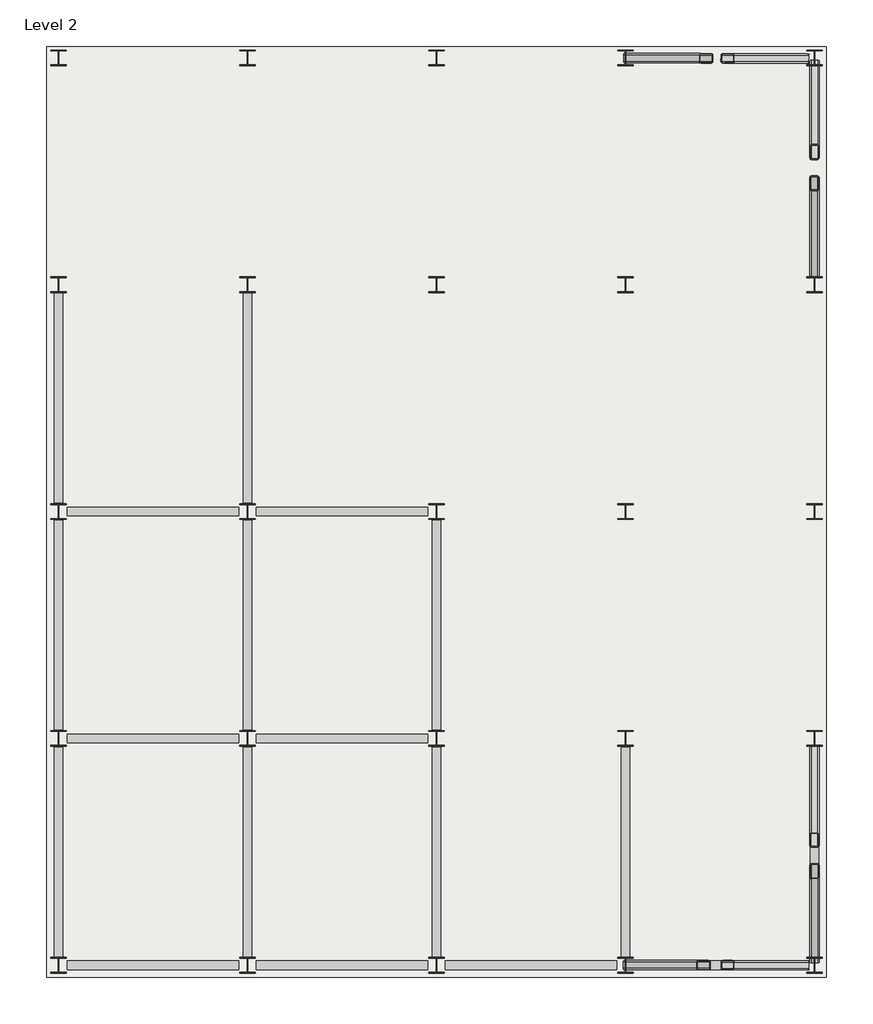
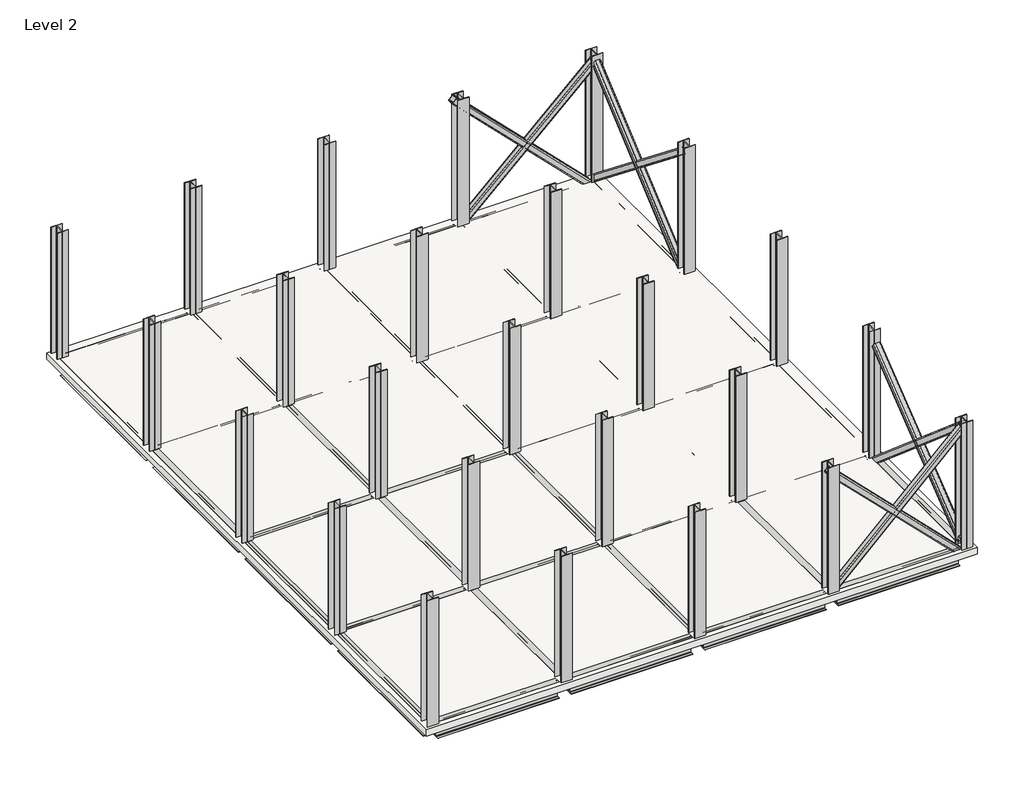
# One storey: 40 beams, 25 columns, 8 members, 1 slab.
"""IFC4 building model written with IfcOpenShell, lengths in millimetres."""

from ifc_helpers import new_model, si_unit, frame, origin, place, context, project, spatial, polyline, outline, extrude, transform, mapped, element, save
from components import w_shapes_w16x26_71b85d0e, w_shapes_w16x26_5730d789, w_shapes_column_w10x49_ceff5d29, hss_square_hss6x6x1_2_008024fe, hss_square_hss6x6x1_2_7c43692b, hss_square_hss6x6x1_2_5f011b37, hss_square_hss6x6x1_2_b9926e2d, hss_square_hss6x6x1_2_e6555cf9, hss_square_hss6x6x1_2_f7a49a43, hss_square_hss6x6x1_2_10b7330d, hss_square_hss6x6x1_2_f3b36863

model = new_model("IFC4")

# Units and contexts
model_context = context("Model", 3, world=origin())
ifc_project = project(units=[si_unit("LENGTHUNIT", "METRE", prefix="MILLI")], contexts=[model_context])

# Site, building, storey
site = spatial("IfcSite", under=ifc_project)
building = spatial("IfcBuilding", under=site)
storey = spatial("IfcBuildingStorey", under=building, Name="Level 2", Elevation=3048.0)

# Beams
placement = place(None, origin())
w_shapes_w16x26_shape = w_shapes_w16x26_71b85d0e(model_context)
element("IfcBeam", 1, ObjectType="W Shapes : W16X26", at=placement, inside=storey, context=model_context, shape_type="MappedRepresentation", body=[
    mapped(w_shapes_w16x26_shape, transform((-5883.5186598, -2213.7239423, 2848.61), x_axis=(1.0, 0.0, 0.0), y_axis=(0.0, 1.0, 0.0), z_axis=(0.0, 0.0, 1.0))),
])
element("IfcBeam", 2, ObjectType="W Shapes : W16X26", at=placement, inside=storey, context=model_context, shape_type="MappedRepresentation", body=[
    mapped(w_shapes_w16x26_shape, transform((-2835.5186598, -2213.7239423, 2848.61), x_axis=(1.0, 0.0, 0.0), y_axis=(0.0, 1.0, 0.0), z_axis=(0.0, 0.0, 1.0))),
])
element("IfcBeam", 3, ObjectType="W Shapes : W16X26", at=placement, inside=storey, context=model_context, shape_type="MappedRepresentation", body=[
    mapped(w_shapes_w16x26_shape, transform((212.4813402, -2213.7239423, 2848.61), x_axis=(1.0, 0.0, 0.0), y_axis=(0.0, 1.0, 0.0), z_axis=(0.0, 0.0, 1.0))),
])
element("IfcBeam", 4, ObjectType="W Shapes : W16X26", at=placement, inside=storey, context=model_context, shape_type="MappedRepresentation", body=[
    mapped(w_shapes_w16x26_shape, transform((3260.4813402, -2213.7239423, 2848.61), x_axis=(1.0, 0.0, 0.0), y_axis=(0.0, 1.0, 0.0), z_axis=(0.0, 0.0, 1.0))),
])
element("IfcBeam", 5, ObjectType="W Shapes : W16X26", at=placement, inside=storey, context=model_context, shape_type="MappedRepresentation", body=[
    mapped(w_shapes_w16x26_shape, transform((-5883.5186598, 1443.8760577, 2848.61), x_axis=(1.0, 0.0, 0.0), y_axis=(0.0, 1.0, 0.0), z_axis=(0.0, 0.0, 1.0))),
])
element("IfcBeam", 6, ObjectType="W Shapes : W16X26", at=placement, inside=storey, context=model_context, shape_type="MappedRepresentation", body=[
    mapped(w_shapes_w16x26_shape, transform((-2835.5186598, 1443.8760577, 2848.61), x_axis=(1.0, 0.0, 0.0), y_axis=(0.0, 1.0, 0.0), z_axis=(0.0, 0.0, 1.0))),
])
element("IfcBeam", 7, ObjectType="W Shapes : W16X26", at=placement, inside=storey, context=model_context, shape_type="MappedRepresentation", body=[
    mapped(w_shapes_w16x26_shape, transform((212.4813402, 1443.8760577, 2848.61), x_axis=(1.0, 0.0, 0.0), y_axis=(0.0, 1.0, 0.0), z_axis=(0.0, 0.0, 1.0))),
])
element("IfcBeam", 8, ObjectType="W Shapes : W16X26", at=placement, inside=storey, context=model_context, shape_type="MappedRepresentation", body=[
    mapped(w_shapes_w16x26_shape, transform((3260.4813402, 1443.8760577, 2848.61), x_axis=(1.0, 0.0, 0.0), y_axis=(0.0, 1.0, 0.0), z_axis=(0.0, 0.0, 1.0))),
])
element("IfcBeam", 9, ObjectType="W Shapes : W16X26", at=placement, inside=storey, context=model_context, shape_type="MappedRepresentation", body=[
    mapped(w_shapes_w16x26_shape, transform((-5883.5186598, 5101.4760577, 2848.61), x_axis=(1.0, 0.0, 0.0), y_axis=(0.0, 1.0, 0.0), z_axis=(0.0, 0.0, 1.0))),
])
element("IfcBeam", 10, ObjectType="W Shapes : W16X26", at=placement, inside=storey, context=model_context, shape_type="MappedRepresentation", body=[
    mapped(w_shapes_w16x26_shape, transform((-2835.5186598, 5101.4760577, 2848.61), x_axis=(1.0, 0.0, 0.0), y_axis=(0.0, 1.0, 0.0), z_axis=(0.0, 0.0, 1.0))),
])
element("IfcBeam", 11, ObjectType="W Shapes : W16X26", at=placement, inside=storey, context=model_context, shape_type="MappedRepresentation", body=[
    mapped(w_shapes_w16x26_shape, transform((212.4813402, 5101.4760577, 2848.61), x_axis=(1.0, 0.0, 0.0), y_axis=(0.0, 1.0, 0.0), z_axis=(0.0, 0.0, 1.0))),
])
element("IfcBeam", 12, ObjectType="W Shapes : W16X26", at=placement, inside=storey, context=model_context, shape_type="MappedRepresentation", body=[
    mapped(w_shapes_w16x26_shape, transform((3260.4813402, 5101.4760577, 2848.61), x_axis=(1.0, 0.0, 0.0), y_axis=(0.0, 1.0, 0.0), z_axis=(0.0, 0.0, 1.0))),
])
element("IfcBeam", 13, ObjectType="W Shapes : W16X26", at=placement, inside=storey, context=model_context, shape_type="MappedRepresentation", body=[
    mapped(w_shapes_w16x26_shape, transform((-5883.5186598, 8759.0760577, 2848.61), x_axis=(1.0, 0.0, 0.0), y_axis=(0.0, 1.0, 0.0), z_axis=(0.0, 0.0, 1.0))),
])
element("IfcBeam", 14, ObjectType="W Shapes : W16X26", at=placement, inside=storey, context=model_context, shape_type="MappedRepresentation", body=[
    mapped(w_shapes_w16x26_shape, transform((-2835.5186598, 8759.0760577, 2848.61), x_axis=(1.0, 0.0, 0.0), y_axis=(0.0, 1.0, 0.0), z_axis=(0.0, 0.0, 1.0))),
])
element("IfcBeam", 15, ObjectType="W Shapes : W16X26", at=placement, inside=storey, context=model_context, shape_type="MappedRepresentation", body=[
    mapped(w_shapes_w16x26_shape, transform((212.4813402, 8759.0760577, 2848.61), x_axis=(1.0, 0.0, 0.0), y_axis=(0.0, 1.0, 0.0), z_axis=(0.0, 0.0, 1.0))),
])
element("IfcBeam", 16, ObjectType="W Shapes : W16X26", at=placement, inside=storey, context=model_context, shape_type="MappedRepresentation", body=[
    mapped(w_shapes_w16x26_shape, transform((3260.4813402, 8759.0760577, 2848.61), x_axis=(1.0, 0.0, 0.0), y_axis=(0.0, 1.0, 0.0), z_axis=(0.0, 0.0, 1.0))),
])
element("IfcBeam", 17, ObjectType="W Shapes : W16X26", at=placement, inside=storey, context=model_context, shape_type="MappedRepresentation", body=[
    mapped(w_shapes_w16x26_shape, transform((-5883.5186598, 12416.6760577, 2848.61), x_axis=(1.0, 0.0, 0.0), y_axis=(0.0, 1.0, 0.0), z_axis=(0.0, 0.0, 1.0))),
])
element("IfcBeam", 18, ObjectType="W Shapes : W16X26", at=placement, inside=storey, context=model_context, shape_type="MappedRepresentation", body=[
    mapped(w_shapes_w16x26_shape, transform((-2835.5186598, 12416.6760577, 2848.61), x_axis=(1.0, 0.0, 0.0), y_axis=(0.0, 1.0, 0.0), z_axis=(0.0, 0.0, 1.0))),
])
element("IfcBeam", 19, ObjectType="W Shapes : W16X26", at=placement, inside=storey, context=model_context, shape_type="MappedRepresentation", body=[
    mapped(w_shapes_w16x26_shape, transform((212.4813402, 12416.6760577, 2848.61), x_axis=(1.0, 0.0, 0.0), y_axis=(0.0, 1.0, 0.0), z_axis=(0.0, 0.0, 1.0))),
])
element("IfcBeam", 20, ObjectType="W Shapes : W16X26", at=placement, inside=storey, context=model_context, shape_type="MappedRepresentation", body=[
    mapped(w_shapes_w16x26_shape, transform((3260.4813402, 12416.6760577, 2848.61), x_axis=(1.0, 0.0, 0.0), y_axis=(0.0, 1.0, 0.0), z_axis=(0.0, 0.0, 1.0))),
])
w_shapes_w16x26_2_shape = w_shapes_w16x26_5730d789(model_context)
element("IfcBeam", 21, ObjectType="W Shapes : W16X26", at=placement, inside=storey, context=model_context, shape_type="MappedRepresentation", body=[
    mapped(w_shapes_w16x26_2_shape, transform((4784.4813402, 10587.8760577, 2848.61), x_axis=(0.0, -1.0, 0.0), y_axis=(1.0, 0.0, 0.0), z_axis=(0.0, 0.0, 1.0))),
])
element("IfcBeam", 22, ObjectType="W Shapes : W16X26", at=placement, inside=storey, context=model_context, shape_type="MappedRepresentation", body=[
    mapped(w_shapes_w16x26_2_shape, transform((4784.4813402, 6930.2760577, 2848.61), x_axis=(0.0, -1.0, 0.0), y_axis=(1.0, 0.0, 0.0), z_axis=(0.0, 0.0, 1.0))),
])
element("IfcBeam", 23, ObjectType="W Shapes : W16X26", at=placement, inside=storey, context=model_context, shape_type="MappedRepresentation", body=[
    mapped(w_shapes_w16x26_2_shape, transform((4784.4813402, 3272.6760577, 2848.61), x_axis=(0.0, -1.0, 0.0), y_axis=(1.0, 0.0, 0.0), z_axis=(0.0, 0.0, 1.0))),
])
element("IfcBeam", 24, ObjectType="W Shapes : W16X26", at=placement, inside=storey, context=model_context, shape_type="MappedRepresentation", body=[
    mapped(w_shapes_w16x26_2_shape, transform((4784.4813402, -384.9239423, 2848.61), x_axis=(0.0, -1.0, 0.0), y_axis=(1.0, 0.0, 0.0), z_axis=(0.0, 0.0, 1.0))),
])
element("IfcBeam", 25, ObjectType="W Shapes : W16X26", at=placement, inside=storey, context=model_context, shape_type="MappedRepresentation", body=[
    mapped(w_shapes_w16x26_2_shape, transform((1736.4813402, 10587.8760577, 2848.61), x_axis=(0.0, -1.0, 0.0), y_axis=(1.0, 0.0, 0.0), z_axis=(0.0, 0.0, 1.0))),
])
element("IfcBeam", 26, ObjectType="W Shapes : W16X26", at=placement, inside=storey, context=model_context, shape_type="MappedRepresentation", body=[
    mapped(w_shapes_w16x26_2_shape, transform((1736.4813402, 6930.2760577, 2848.61), x_axis=(0.0, -1.0, 0.0), y_axis=(1.0, 0.0, 0.0), z_axis=(0.0, 0.0, 1.0))),
])
element("IfcBeam", 27, ObjectType="W Shapes : W16X26", at=placement, inside=storey, context=model_context, shape_type="MappedRepresentation", body=[
    mapped(w_shapes_w16x26_2_shape, transform((1736.4813402, 3272.6760577, 2848.61), x_axis=(0.0, -1.0, 0.0), y_axis=(1.0, 0.0, 0.0), z_axis=(0.0, 0.0, 1.0))),
])
element("IfcBeam", 28, ObjectType="W Shapes : W16X26", at=placement, inside=storey, context=model_context, shape_type="MappedRepresentation", body=[
    mapped(w_shapes_w16x26_2_shape, transform((1736.4813402, -384.9239423, 2848.61), x_axis=(0.0, -1.0, 0.0), y_axis=(1.0, 0.0, 0.0), z_axis=(0.0, 0.0, 1.0))),
])
element("IfcBeam", 29, ObjectType="W Shapes : W16X26", at=placement, inside=storey, context=model_context, shape_type="MappedRepresentation", body=[
    mapped(w_shapes_w16x26_2_shape, transform((-1311.5186598, 10587.8760577, 2848.61), x_axis=(0.0, -1.0, 0.0), y_axis=(1.0, 0.0, 0.0), z_axis=(0.0, 0.0, 1.0))),
])
element("IfcBeam", 30, ObjectType="W Shapes : W16X26", at=placement, inside=storey, context=model_context, shape_type="MappedRepresentation", body=[
    mapped(w_shapes_w16x26_2_shape, transform((-1311.5186598, 6930.2760577, 2848.61), x_axis=(0.0, -1.0, 0.0), y_axis=(1.0, 0.0, 0.0), z_axis=(0.0, 0.0, 1.0))),
])
element("IfcBeam", 31, ObjectType="W Shapes : W16X26", at=placement, inside=storey, context=model_context, shape_type="MappedRepresentation", body=[
    mapped(w_shapes_w16x26_2_shape, transform((-1311.5186598, 3272.6760577, 2848.61), x_axis=(0.0, -1.0, 0.0), y_axis=(1.0, 0.0, 0.0), z_axis=(0.0, 0.0, 1.0))),
])
element("IfcBeam", 32, ObjectType="W Shapes : W16X26", at=placement, inside=storey, context=model_context, shape_type="MappedRepresentation", body=[
    mapped(w_shapes_w16x26_2_shape, transform((-1311.5186598, -384.9239423, 2848.61), x_axis=(0.0, -1.0, 0.0), y_axis=(1.0, 0.0, 0.0), z_axis=(0.0, 0.0, 1.0))),
])
element("IfcBeam", 33, ObjectType="W Shapes : W16X26", at=placement, inside=storey, context=model_context, shape_type="MappedRepresentation", body=[
    mapped(w_shapes_w16x26_2_shape, transform((-4359.5186598, 10587.8760577, 2848.61), x_axis=(0.0, -1.0, 0.0), y_axis=(1.0, 0.0, 0.0), z_axis=(0.0, 0.0, 1.0))),
])
element("IfcBeam", 34, ObjectType="W Shapes : W16X26", at=placement, inside=storey, context=model_context, shape_type="MappedRepresentation", body=[
    mapped(w_shapes_w16x26_2_shape, transform((-4359.5186598, 6930.2760577, 2848.61), x_axis=(0.0, -1.0, 0.0), y_axis=(1.0, 0.0, 0.0), z_axis=(0.0, 0.0, 1.0))),
])
element("IfcBeam", 35, ObjectType="W Shapes : W16X26", at=placement, inside=storey, context=model_context, shape_type="MappedRepresentation", body=[
    mapped(w_shapes_w16x26_2_shape, transform((-4359.5186598, 3272.6760577, 2848.61), x_axis=(0.0, -1.0, 0.0), y_axis=(1.0, 0.0, 0.0), z_axis=(0.0, 0.0, 1.0))),
])
element("IfcBeam", 36, ObjectType="W Shapes : W16X26", at=placement, inside=storey, context=model_context, shape_type="MappedRepresentation", body=[
    mapped(w_shapes_w16x26_2_shape, transform((-4359.5186598, -384.9239423, 2848.61), x_axis=(0.0, -1.0, 0.0), y_axis=(1.0, 0.0, 0.0), z_axis=(0.0, 0.0, 1.0))),
])
element("IfcBeam", 37, ObjectType="W Shapes : W16X26", at=placement, inside=storey, context=model_context, shape_type="MappedRepresentation", body=[
    mapped(w_shapes_w16x26_2_shape, transform((-7407.5186598, 10587.8760577, 2848.61), x_axis=(0.0, -1.0, 0.0), y_axis=(1.0, 0.0, 0.0), z_axis=(0.0, 0.0, 1.0))),
])
element("IfcBeam", 38, ObjectType="W Shapes : W16X26", at=placement, inside=storey, context=model_context, shape_type="MappedRepresentation", body=[
    mapped(w_shapes_w16x26_2_shape, transform((-7407.5186598, 6930.2760577, 2848.61), x_axis=(0.0, -1.0, 0.0), y_axis=(1.0, 0.0, 0.0), z_axis=(0.0, 0.0, 1.0))),
])
element("IfcBeam", 39, ObjectType="W Shapes : W16X26", at=placement, inside=storey, context=model_context, shape_type="MappedRepresentation", body=[
    mapped(w_shapes_w16x26_2_shape, transform((-7407.5186598, 3272.6760577, 2848.61), x_axis=(0.0, -1.0, 0.0), y_axis=(1.0, 0.0, 0.0), z_axis=(0.0, 0.0, 1.0))),
])
element("IfcBeam", 40, ObjectType="W Shapes : W16X26", at=placement, inside=storey, context=model_context, shape_type="MappedRepresentation", body=[
    mapped(w_shapes_w16x26_2_shape, transform((-7407.5186598, -384.9239423, 2848.61), x_axis=(0.0, -1.0, 0.0), y_axis=(1.0, 0.0, 0.0), z_axis=(0.0, 0.0, 1.0))),
])

# Columns
w_shapes_column_w10x49_shape = w_shapes_column_w10x49_ceff5d29(model_context)
element("IfcColumn", 41, ObjectType="W Shapes-Column : W10X49", at=placement, inside=storey, context=model_context, shape_type="MappedRepresentation", body=[
    mapped(w_shapes_column_w10x49_shape, transform((4784.4813402, -2213.7239423, 0.0), x_axis=(1.0, 0.0, 0.0), y_axis=(0.0, 1.0, 0.0), z_axis=(0.0, 0.0, 1.0))),
])
element("IfcColumn", 42, ObjectType="W Shapes-Column : W10X49", at=placement, inside=storey, context=model_context, shape_type="MappedRepresentation", body=[
    mapped(w_shapes_column_w10x49_shape, transform((1736.4813402, -2213.7239423, 0.0), x_axis=(1.0, 0.0, 0.0), y_axis=(0.0, 1.0, 0.0), z_axis=(0.0, 0.0, 1.0))),
])
element("IfcColumn", 43, ObjectType="W Shapes-Column : W10X49", at=placement, inside=storey, context=model_context, shape_type="MappedRepresentation", body=[
    mapped(w_shapes_column_w10x49_shape, transform((-1311.5186598, -2213.7239423, 0.0), x_axis=(1.0, 0.0, 0.0), y_axis=(0.0, 1.0, 0.0), z_axis=(0.0, 0.0, 1.0))),
])
element("IfcColumn", 44, ObjectType="W Shapes-Column : W10X49", at=placement, inside=storey, context=model_context, shape_type="MappedRepresentation", body=[
    mapped(w_shapes_column_w10x49_shape, transform((-4359.5186598, -2213.7239423, 0.0), x_axis=(1.0, 0.0, 0.0), y_axis=(0.0, 1.0, 0.0), z_axis=(0.0, 0.0, 1.0))),
])
element("IfcColumn", 45, ObjectType="W Shapes-Column : W10X49", at=placement, inside=storey, context=model_context, shape_type="MappedRepresentation", body=[
    mapped(w_shapes_column_w10x49_shape, transform((-7407.5186598, -2213.7239423, 0.0), x_axis=(1.0, 0.0, 0.0), y_axis=(0.0, 1.0, 0.0), z_axis=(0.0, 0.0, 1.0))),
])
element("IfcColumn", 46, ObjectType="W Shapes-Column : W10X49", at=placement, inside=storey, context=model_context, shape_type="MappedRepresentation", body=[
    mapped(w_shapes_column_w10x49_shape, transform((4784.4813402, 1443.8760577, 0.0), x_axis=(1.0, 0.0, 0.0), y_axis=(0.0, 1.0, 0.0), z_axis=(0.0, 0.0, 1.0))),
])
element("IfcColumn", 47, ObjectType="W Shapes-Column : W10X49", at=placement, inside=storey, context=model_context, shape_type="MappedRepresentation", body=[
    mapped(w_shapes_column_w10x49_shape, transform((4784.4813402, 5101.4760577, 0.0), x_axis=(1.0, 0.0, 0.0), y_axis=(0.0, 1.0, 0.0), z_axis=(0.0, 0.0, 1.0))),
])
element("IfcColumn", 48, ObjectType="W Shapes-Column : W10X49", at=placement, inside=storey, context=model_context, shape_type="MappedRepresentation", body=[
    mapped(w_shapes_column_w10x49_shape, transform((4784.4813402, 8759.0760577, 0.0), x_axis=(1.0, 0.0, 0.0), y_axis=(0.0, 1.0, 0.0), z_axis=(0.0, 0.0, 1.0))),
])
element("IfcColumn", 49, ObjectType="W Shapes-Column : W10X49", at=placement, inside=storey, context=model_context, shape_type="MappedRepresentation", body=[
    mapped(w_shapes_column_w10x49_shape, transform((4784.4813402, 12416.6760577, 0.0), x_axis=(1.0, 0.0, 0.0), y_axis=(0.0, 1.0, 0.0), z_axis=(0.0, 0.0, 1.0))),
])
element("IfcColumn", 50, ObjectType="W Shapes-Column : W10X49", at=placement, inside=storey, context=model_context, shape_type="MappedRepresentation", body=[
    mapped(w_shapes_column_w10x49_shape, transform((1736.4813402, 1443.8760577, 0.0), x_axis=(1.0, 0.0, 0.0), y_axis=(0.0, 1.0, 0.0), z_axis=(0.0, 0.0, 1.0))),
])
element("IfcColumn", 51, ObjectType="W Shapes-Column : W10X49", at=placement, inside=storey, context=model_context, shape_type="MappedRepresentation", body=[
    mapped(w_shapes_column_w10x49_shape, transform((-1311.5186598, 1443.8760577, 0.0), x_axis=(1.0, 0.0, 0.0), y_axis=(0.0, 1.0, 0.0), z_axis=(0.0, 0.0, 1.0))),
])
element("IfcColumn", 52, ObjectType="W Shapes-Column : W10X49", at=placement, inside=storey, context=model_context, shape_type="MappedRepresentation", body=[
    mapped(w_shapes_column_w10x49_shape, transform((-4359.5186598, 1443.8760577, 0.0), x_axis=(1.0, 0.0, 0.0), y_axis=(0.0, 1.0, 0.0), z_axis=(0.0, 0.0, 1.0))),
])
element("IfcColumn", 53, ObjectType="W Shapes-Column : W10X49", at=placement, inside=storey, context=model_context, shape_type="MappedRepresentation", body=[
    mapped(w_shapes_column_w10x49_shape, transform((-7407.5186598, 1443.8760577, 0.0), x_axis=(1.0, 0.0, 0.0), y_axis=(0.0, 1.0, 0.0), z_axis=(0.0, 0.0, 1.0))),
])
element("IfcColumn", 54, ObjectType="W Shapes-Column : W10X49", at=placement, inside=storey, context=model_context, shape_type="MappedRepresentation", body=[
    mapped(w_shapes_column_w10x49_shape, transform((1736.4813402, 5101.4760577, 0.0), x_axis=(1.0, 0.0, 0.0), y_axis=(0.0, 1.0, 0.0), z_axis=(0.0, 0.0, 1.0))),
])
element("IfcColumn", 55, ObjectType="W Shapes-Column : W10X49", at=placement, inside=storey, context=model_context, shape_type="MappedRepresentation", body=[
    mapped(w_shapes_column_w10x49_shape, transform((-1311.5186598, 5101.4760577, 0.0), x_axis=(1.0, 0.0, 0.0), y_axis=(0.0, 1.0, 0.0), z_axis=(0.0, 0.0, 1.0))),
])
element("IfcColumn", 56, ObjectType="W Shapes-Column : W10X49", at=placement, inside=storey, context=model_context, shape_type="MappedRepresentation", body=[
    mapped(w_shapes_column_w10x49_shape, transform((-4359.5186598, 5101.4760577, 0.0), x_axis=(1.0, 0.0, 0.0), y_axis=(0.0, 1.0, 0.0), z_axis=(0.0, 0.0, 1.0))),
])
element("IfcColumn", 57, ObjectType="W Shapes-Column : W10X49", at=placement, inside=storey, context=model_context, shape_type="MappedRepresentation", body=[
    mapped(w_shapes_column_w10x49_shape, transform((-7407.5186598, 5101.4760577, 0.0), x_axis=(1.0, 0.0, 0.0), y_axis=(0.0, 1.0, 0.0), z_axis=(0.0, 0.0, 1.0))),
])
element("IfcColumn", 58, ObjectType="W Shapes-Column : W10X49", at=placement, inside=storey, context=model_context, shape_type="MappedRepresentation", body=[
    mapped(w_shapes_column_w10x49_shape, transform((1736.4813402, 8759.0760577, 0.0), x_axis=(1.0, 0.0, 0.0), y_axis=(0.0, 1.0, 0.0), z_axis=(0.0, 0.0, 1.0))),
])
element("IfcColumn", 59, ObjectType="W Shapes-Column : W10X49", at=placement, inside=storey, context=model_context, shape_type="MappedRepresentation", body=[
    mapped(w_shapes_column_w10x49_shape, transform((-1311.5186598, 8759.0760577, 0.0), x_axis=(1.0, 0.0, 0.0), y_axis=(0.0, 1.0, 0.0), z_axis=(0.0, 0.0, 1.0))),
])
element("IfcColumn", 60, ObjectType="W Shapes-Column : W10X49", at=placement, inside=storey, context=model_context, shape_type="MappedRepresentation", body=[
    mapped(w_shapes_column_w10x49_shape, transform((-4359.5186598, 8759.0760577, 0.0), x_axis=(1.0, 0.0, 0.0), y_axis=(0.0, 1.0, 0.0), z_axis=(0.0, 0.0, 1.0))),
])
element("IfcColumn", 61, ObjectType="W Shapes-Column : W10X49", at=placement, inside=storey, context=model_context, shape_type="MappedRepresentation", body=[
    mapped(w_shapes_column_w10x49_shape, transform((-7407.5186598, 8759.0760577, 0.0), x_axis=(1.0, 0.0, 0.0), y_axis=(0.0, 1.0, 0.0), z_axis=(0.0, 0.0, 1.0))),
])
element("IfcColumn", 62, ObjectType="W Shapes-Column : W10X49", at=placement, inside=storey, context=model_context, shape_type="MappedRepresentation", body=[
    mapped(w_shapes_column_w10x49_shape, transform((1736.4813402, 12416.6760577, 0.0), x_axis=(1.0, 0.0, 0.0), y_axis=(0.0, 1.0, 0.0), z_axis=(0.0, 0.0, 1.0))),
])
element("IfcColumn", 63, ObjectType="W Shapes-Column : W10X49", at=placement, inside=storey, context=model_context, shape_type="MappedRepresentation", body=[
    mapped(w_shapes_column_w10x49_shape, transform((-1311.5186598, 12416.6760577, 0.0), x_axis=(1.0, 0.0, 0.0), y_axis=(0.0, 1.0, 0.0), z_axis=(0.0, 0.0, 1.0))),
])
element("IfcColumn", 64, ObjectType="W Shapes-Column : W10X49", at=placement, inside=storey, context=model_context, shape_type="MappedRepresentation", body=[
    mapped(w_shapes_column_w10x49_shape, transform((-4359.5186598, 12416.6760577, 0.0), x_axis=(1.0, 0.0, 0.0), y_axis=(0.0, 1.0, 0.0), z_axis=(0.0, 0.0, 1.0))),
])
element("IfcColumn", 65, ObjectType="W Shapes-Column : W10X49", at=placement, inside=storey, context=model_context, shape_type="MappedRepresentation", body=[
    mapped(w_shapes_column_w10x49_shape, transform((-7407.5186598, 12416.6760577, 0.0), x_axis=(1.0, 0.0, 0.0), y_axis=(0.0, 1.0, 0.0), z_axis=(0.0, 0.0, 1.0))),
])

# Members
hss_square_hss6x6x1_2_shape = hss_square_hss6x6x1_2_008024fe(model_context)
element("IfcMember", 66, ObjectType="HSS Square : HSS6X6X1/2", at=placement, inside=storey, context=model_context, shape_type="MappedRepresentation", body=[
    mapped(hss_square_hss6x6x1_2_shape, transform((4784.4813402, 10587.8760577, 4495.8), x_axis=(0.0, 0.7840458244617616, -0.6207029443655613), y_axis=(-1.0000000000000002, 0.0, 0.0), z_axis=(0.0, 0.6207029443655613, 0.7840458244617616))),
])
hss_square_hss6x6x1_2_2_shape = hss_square_hss6x6x1_2_7c43692b(model_context)
element("IfcMember", 67, ObjectType="HSS Square : HSS6X6X1/2", at=placement, inside=storey, context=model_context, shape_type="MappedRepresentation", body=[
    mapped(hss_square_hss6x6x1_2_2_shape, transform((4784.4813402, 10587.8760577, 4412.1631022), x_axis=(0.0, -0.760075346032819, -0.6498349547024158), y_axis=(1.0000000000000002, 0.0, 0.0), z_axis=(0.0, -0.6498349547024158, 0.760075346032819))),
])
hss_square_hss6x6x1_2_3_shape = hss_square_hss6x6x1_2_5f011b37(model_context)
element("IfcMember", 68, ObjectType="HSS Square : HSS6X6X1/2", at=placement, inside=storey, context=model_context, shape_type="MappedRepresentation", body=[
    mapped(hss_square_hss6x6x1_2_3_shape, transform((4784.4813402, -384.9239423, 4412.1631022), x_axis=(0.0, 0.7600753460328191, -0.6498349547024159), y_axis=(-1.0000000000000002, 0.0, 0.0), z_axis=(0.0, 0.6498349547024159, 0.7600753460328191))),
])
hss_square_hss6x6x1_2_4_shape = hss_square_hss6x6x1_2_b9926e2d(model_context)
element("IfcMember", 69, ObjectType="HSS Square : HSS6X6X1/2", at=placement, inside=storey, context=model_context, shape_type="MappedRepresentation", body=[
    mapped(hss_square_hss6x6x1_2_4_shape, transform((4784.4813402, -384.9239423, 4495.8), x_axis=(0.0, -0.7840458244617616, -0.6207029443655613), y_axis=(1.0000000000000002, 0.0, 0.0), z_axis=(0.0, -0.6207029443655613, 0.7840458244617616))),
])
hss_square_hss6x6x1_2_5_shape = hss_square_hss6x6x1_2_e6555cf9(model_context)
element("IfcMember", 70, ObjectType="HSS Square : HSS6X6X1/2", at=placement, inside=storey, context=model_context, shape_type="MappedRepresentation", body=[
    mapped(hss_square_hss6x6x1_2_5_shape, transform((3168.0352384, -2213.7239423, 4413.8521986), x_axis=(-0.718393447364439, 0.0, -0.6956370136672122), y_axis=(0.0, -1.0000000000000002, 0.0), z_axis=(-0.6956370136672122, 0.0, 0.718393447364439))),
])
hss_square_hss6x6x1_2_6_shape = hss_square_hss6x6x1_2_f7a49a43(model_context)
element("IfcMember", 71, ObjectType="HSS Square : HSS6X6X1/2", at=placement, inside=storey, context=model_context, shape_type="MappedRepresentation", body=[
    mapped(hss_square_hss6x6x1_2_6_shape, transform((3260.4813402, -2213.7239423, 4372.61), x_axis=(0.7071067811865475, 0.0, -0.7071067811865477), y_axis=(0.0, 1.0000000000000002, 0.0), z_axis=(0.7071067811865477, 0.0, 0.7071067811865475))),
])
hss_square_hss6x6x1_2_7_shape = hss_square_hss6x6x1_2_10b7330d(model_context)
element("IfcMember", 72, ObjectType="HSS Square : HSS6X6X1/2", at=placement, inside=storey, context=model_context, shape_type="MappedRepresentation", body=[
    mapped(hss_square_hss6x6x1_2_7_shape, transform((3168.0352384, 12409.9819642, 4372.61), x_axis=(-0.7276035720332941, 0.003013182054487383, -0.6859912264003803), y_axis=(-0.004141205915939178, -0.9999914251700173, 0.0), z_axis=(-0.6859853441422442, 0.002840830925050774, 0.7276098111637187))),
])
hss_square_hss6x6x1_2_8_shape = hss_square_hss6x6x1_2_f3b36863(model_context)
element("IfcMember", 73, ObjectType="HSS Square : HSS6X6X1/2", at=placement, inside=storey, context=model_context, shape_type="MappedRepresentation", body=[
    mapped(hss_square_hss6x6x1_2_8_shape, transform((3260.4813402, 12409.9819642, 4372.61), x_axis=(0.7071033705496137, -0.0031059160887349836, -0.7071033705496146), y_axis=(0.004392407470180804, 0.9999903533317791, 0.0), z_axis=(0.7070965493580008, -0.003105886126991347, 0.7071101918070298))),
])

# Slab
element("IfcSlab", 74, ObjectType="6\" Foundation Slab", at=placement, inside=storey, context=model_context, shape_type="SweptSolid", body=[
    extrude(outline(polyline([(4974.3230176, 12600.4819642), (4974.3230176, -2410.9180358), (-7598.6769824, -2410.9180358), (-7598.6769824, 12600.4819642), (4974.3230176, 12600.4819642)])), frame((0.0, 0.0, 2895.6), z_axis=(0.0, 0.0, 1.0), x_axis=(1.0, 0.0, 0.0)), (0.0, 0.0, 1.0), 152.4),
])

save(model, "model.ifc")

# Revit data of these elements
# Type "W Shapes : W16X26"
#   Section Name Key = "W16x26"
#   Assembly Code = "B10"
#   Width = 5.500"
#   Web Thickness = 0.250"
#   Web Fillet = 0.402"
#   Warping Constant = 565.00 in⁶
#   Torsional Moment of Inertia = 0.262 in⁴
#   Section Area = 7.68 in²
#   Plastic Modulus weak axis = 5.48 in³
#   Plastic Modulus strong axis = 44.20 in³
#   Perimeter = 52.20 ft²/ft
#   Nominal Weight = 26.00 lbf/ft
#   Moment of Inertia weak axis = 9.59 in⁴
#   Moment of Inertia strong axis = 301.00 in⁴
#   Height = 15.700"
#   Flange Thickness = 0.345"
#   Elastic Modulus weak axis = 3.49 in³
#   Elastic Modulus strong axis = 38.40 in³
#   Centroid Vertical = 7.850"
#   Centroid Horizontal = 2.750"
#   Bolt Spacing = 0' - 3 1/2"
#   Length [instance default] = 5' - 0"
#   Structural Material [instance default] = Steel ASTM A992
#   Principal Axes Angle = 0
# Type "W Shapes-Column : W10X49"
#   Section Name Key = "W10x49"
#   Assembly Code = "B10"
#   Width = 10.000"
#   Web Thickness = 0.340"
#   Web Fillet = 0.500"
#   Warping Constant = 2070.00 in⁶
#   Torsional Moment of Inertia = 1.39 in⁴
#   Section Area = 14.40 in²
#   Plastic Modulus weak axis = 28.30 in³
#   Plastic Modulus strong axis = 60.40 in³
#   Perimeter = 58.50 ft²/ft
#   Nominal Weight = 49.00 lbf/ft
#   Moment of Inertia weak axis = 93.40 in⁴
#   Moment of Inertia strong axis = 272.00 in⁴
#   Height = 10.000"
#   Flange Thickness = 0.560"
#   Elastic Modulus weak axis = 18.70 in³
#   Elastic Modulus strong axis = 54.60 in³
#   Centroid Vertical = 5.000"
#   Centroid Horizontal = 5.000"
#   Bolt Spacing = 0' - 5 1/2"
#   Structural Material [instance default] = Steel ASTM A992
#   Principal Axes Angle = 0
# Type "HSS Square : HSS6X6X1/2"
#   Section Name Key = "HSS 6X6X1/2"
#   Assembly Code = "B10"
#   Width = 6.000"
#   Wall Nominal Thickness = 0.500"
#   Wall Design Thickness = 0.465"
#   Torsional Moment of Inertia = 81.10 in⁴
#   Torsional Modulus = 28.10 in³
#   Section Area = 9.74 in²
#   Plastic Modulus weak axis = 19.80 in³
#   Plastic Modulus strong axis = 19.80 in³
#   Outer Fillet = 1.000"
#   Nominal Weight = 35.24 lbf/ft
#   Moment of Inertia weak axis = 48.30 in⁴
#   Moment of Inertia strong axis = 48.30 in⁴
#   Inner Fillet = 0.500"
#   Height = 6.000"
#   Elastic Modulus weak axis = 16.10 in³
#   Elastic Modulus strong axis = 16.10 in³
#   Centroid Vertical = 3.000"
#   Centroid Horizontal = 3.000"
#   Length [instance default] = 5' - 0"
#   Structural Material [instance default] = Steel ASTM A500, Grade B, Rectangular and Square
#   Principal Axes Angle = 0
# Type "6\" Foundation Slab"
#   Layers, outside or top first: 0' - 6" "Concrete, Cast-in-Place gray" (function 1)
# Elements 1, 2, 3, 4, 5, 6, 7, 8, 9, 10, 11, 12, 13, 14, 15, 16, 17, 18, 19, 20, 21, 22, 23, 24, 25, 26, 27, 28, 29, 30, 31, 32, 33, 34, 35, 36, 37, 38, 39, 40 (IfcBeam, "W Shapes : W16X26")
#   Comments = ""
#   Structural Material = Steel ASTM A992
#   Phase Created = New Construction
#   Materials on its faces: "Steel ASTM A992"
# Elements 41, 42, 43, 44, 45, 46, 47, 48, 49, 50, 51, 52, 53, 54, 55, 56, 57, 58, 59, 60, 61, 62, 63, 64, 65 (IfcColumn, "W Shapes-Column : W10X49")
#   Structural Material = Steel ASTM A992
#   Phase Created = New Construction
#   Materials on its faces: "Steel ASTM A992"
# Elements 66, 67, 68, 69, 70, 71, 72, 73 (IfcMember, "HSS Square : HSS6X6X1/2")
#   Comments = ""
#   Structural Material = Steel ASTM A992
#   Phase Created = New Construction
#   Materials on its faces: "Steel ASTM A992"
# Element 74 (IfcSlab, "6\" Foundation Slab")
#   Height Offset From Level = 0' - 0"
#   built-in parameter 1001954 = 1
#   Phase Created = New Construction
#   Materials on its faces: "Concrete, Cast-in-Place gray"
# Materials
#   "Steel ASTM A992": class "Metal", colour RGB 199 199 199, transparency 0, Description = "Structural steel 50ksi", Cost = 0
#   "Steel ASTM A500, Grade B, Rectangular and Square": class "Metal", colour RGB 199 199 199, transparency 0, Description = "Carbon steel", Cost = 0
#   "Concrete, Cast-in-Place gray": class "Concrete", colour RGB 192 192 192, transparency 0, Description = "Cast-in-place concrete", Cost = 0
